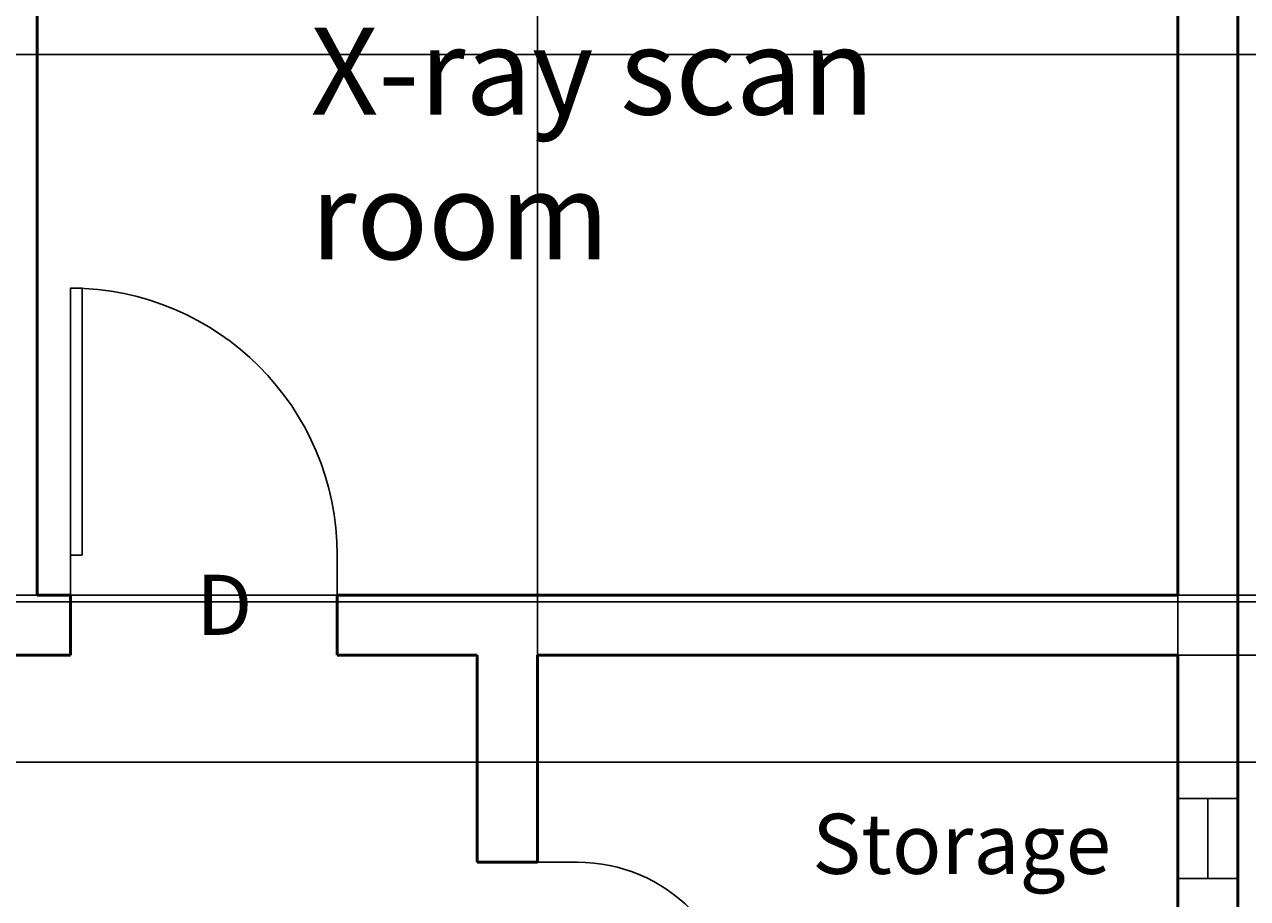
# Model space of a CAD drawing. Units: inches. Extents: x -364 to 705, y -52 to 1250.
# Tile 31 of 34: x 366 to 549, y 786 to 917. Entities that reach past the tile are written whole.
import ezdxf

# ---------------------------------------------------------------- set-up
doc = ezdxf.new("R2010")
doc.units = ezdxf.units.IN
doc.header["$MEASUREMENT"] = 0
for name, color, linetype, lineweight in [('A-ANNO-DIMS', 4, 'Continuous', 18), ('A-ANNO-IDEN', 1, 'Continuous', 18), ('A-AREA-IDEN', 3, 'Continuous', 18), ('A-DOOR', 1, 'Continuous', 25), ('A-GLAZ', 4, 'Continuous', 25), ('A-WALL', 41, 'Continuous', 50)]:
    doc.layers.add(name, color=color, linetype=linetype, lineweight=lineweight)
doc.styles.get("Standard").update_dxf_attribs({"font": 'arial.ttf'})
doc.dimstyles.get("Standard").update_dxf_attribs({"dimtxt": 1, "dimasz": 1, "dimexe": 0.18, "dimexo": 0.0625, "dimgap": 0.09, "dimtad": 0, "dimtih": 1, "dimtoh": 1, "dimdec": 0, "dimzin": 0, "dimdsep": 46, "dimlunit": 3, "dimtxsty": 'Standard', "dimcen": 0.09, "dimadec": 0, "dimazin": 0, "dimtfac": 1, "dimtdec": 0, "dimtofl": 0, "dimtmove": 0, "dimatfit": 3, "dimfxl": 1, "dimtolj": 1, "dimtzin": 0, "dimarcsym": 0})

# ---------------------------------------------------------------- blocks, each defined once
blk = doc.blocks.new('*U2')
for p, q in [((0, 0), (0, -6)), ((40, 0), (40, -6))]:
    blk.add_line(p, q)
blk.add_lwpolyline([(0, 0), (0, 40), (1.75, 40), (1.75, 0)], close=True)
blk.add_arc((0, 0), 40, 0, 90)
blk = doc.blocks.new('*U3')
for p, q in [((0, 0), (0, -6)), ((-24, 0), (-24, -6))]:
    blk.add_line(p, q)
blk.add_lwpolyline([(0, 0), (0, 24), (-1.75, 24), (-1.75, 0)], close=True)
blk.add_arc((0, 0), 24, 90, 180)
blk = doc.blocks.new('*D83')
at = {"layer": 'A-ANNO-DIMS', "color": 0, "lineweight": -2, "transparency": 16777216}
for p, q in [((538.64, 822.11), (703.01, 822.11)), ((702.83, 821.11), (702.83, 788.22)), ((702.83, 754.11), (702.83, 787.01)), ((538.64, 753.11), (703.01, 753.11))]:
    blk.add_line(p, q, dxfattribs=at)
at = {"layer": 'A-ANNO-DIMS', "color": 0, "transparency": 16777216}
for points in [[(702.66, 821.11), (703, 821.11), (702.83, 822.11)], [(702.66, 754.11), (703, 754.11), (702.83, 753.11)]]:
    blk.add_solid(points, dxfattribs=at)
at = {"layer": 'Defpoints', "color": 0, "transparency": 16777216}
for p in [(538.58, 822.11), (702.83, 822.11), (538.58, 753.11)]:
    blk.add_point(p, dxfattribs=at)
at = {"layer": 'A-ANNO-DIMS', "color": 0, "transparency": 16777216, "insert": (702.83, 787.61), "char_height": 1, "attachment_point": 5}
blk.add_mtext('\\A1;5\'-9"', dxfattribs=at)
blk = doc.blocks.new('*D84')
at = {"layer": 'A-ANNO-DIMS', "color": 0, "lineweight": -2, "transparency": 16777216}
for p, q in [((547.64, 986.11), (703.01, 986.11)), ((702.83, 985.11), (702.83, 904.72)), ((702.83, 823.11), (702.83, 903.51)), ((538.64, 822.11), (703.01, 822.11))]:
    blk.add_line(p, q, dxfattribs=at)
at = {"layer": 'A-ANNO-DIMS', "color": 0, "transparency": 16777216}
for points in [[(702.66, 985.11), (703, 985.11), (702.83, 986.11)], [(702.66, 823.11), (703, 823.11), (702.83, 822.11)]]:
    blk.add_solid(points, dxfattribs=at)
at = {"layer": 'Defpoints', "color": 0, "transparency": 16777216}
for p in [(547.58, 986.11), (702.83, 986.11), (538.58, 822.11)]:
    blk.add_point(p, dxfattribs=at)
at = {"layer": 'A-ANNO-DIMS', "color": 0, "transparency": 16777216, "insert": (702.83, 904.11), "char_height": 1, "attachment_point": 5}
blk.add_mtext('\\A1;13\'-8"', dxfattribs=at)
blk = doc.blocks.new('*D97')
at = {"layer": 'A-ANNO-DIMS', "color": 0, "lineweight": -2, "transparency": 16777216}
for p, q in [((358.64, 912.11), (703.01, 912.11)), ((702.83, 911.11), (702.83, 872.22)), ((702.83, 832.11), (702.83, 871.01)), ((358.64, 831.11), (703.01, 831.11))]:
    blk.add_line(p, q, dxfattribs=at)
at = {"layer": 'A-ANNO-DIMS', "color": 0, "transparency": 16777216}
for points in [[(702.66, 911.11), (703, 911.11), (702.83, 912.11)], [(702.66, 832.11), (703, 832.11), (702.83, 831.11)]]:
    blk.add_solid(points, dxfattribs=at)
at = {"layer": 'Defpoints', "color": 0, "transparency": 16777216}
for p in [(358.58, 912.11), (358.58, 831.11), (702.83, 831.11)]:
    blk.add_point(p, dxfattribs=at)
at = {"layer": 'A-ANNO-DIMS', "color": 0, "transparency": 16777216, "insert": (702.83, 871.61), "char_height": 1, "attachment_point": 5}
blk.add_mtext('\\A1;6\'-9"', dxfattribs=at)
blk = doc.blocks.new('*D99')
at = {"layer": 'A-ANNO-DIMS', "color": 0, "lineweight": -2, "transparency": 16777216}
for p, q in [((442.58, 822.18), (442.58, 1141.54)), ((443.58, 1141.36), (489.16, 1141.36)), ((537.58, 1141.36), (492, 1141.36)), ((538.58, 822.18), (538.58, 1141.54))]:
    blk.add_line(p, q, dxfattribs=at)
at = {"layer": 'A-ANNO-DIMS', "color": 0, "transparency": 16777216}
for points in [[(443.58, 1141.53), (443.58, 1141.2), (442.58, 1141.36)], [(537.58, 1141.53), (537.58, 1141.2), (538.58, 1141.36)]]:
    blk.add_solid(points, dxfattribs=at)
at = {"layer": 'Defpoints', "color": 0, "transparency": 16777216}
for p in [(538.58, 1141.36), (442.58, 822.11), (538.58, 822.11)]:
    blk.add_point(p, dxfattribs=at)
at = {"layer": 'A-ANNO-DIMS', "color": 0, "transparency": 16777216, "insert": (490.58, 1141.36), "char_height": 1, "attachment_point": 5}
blk.add_mtext('\\A1;8\'-0"', dxfattribs=at)
blk = doc.blocks.new('*D105')
at = {"layer": 'A-ANNO-DIMS', "color": 0, "lineweight": -2, "transparency": 16777216}
for p, q in [((148.64, 830.11), (703.01, 830.11)), ((702.83, 829.11), (702.83, 818.72)), ((702.83, 807.11), (702.83, 817.51)), ((148.64, 806.11), (703.01, 806.11))]:
    blk.add_line(p, q, dxfattribs=at)
at = {"layer": 'A-ANNO-DIMS', "color": 0, "transparency": 16777216}
for points in [[(702.66, 829.11), (703, 829.11), (702.83, 830.11)], [(702.66, 807.11), (703, 807.11), (702.83, 806.11)]]:
    blk.add_solid(points, dxfattribs=at)
at = {"layer": 'Defpoints', "color": 0, "transparency": 16777216}
for p in [(148.58, 830.11), (148.58, 806.11), (702.83, 806.11)]:
    blk.add_point(p, dxfattribs=at)
at = {"layer": 'A-ANNO-DIMS', "color": 0, "transparency": 16777216, "insert": (702.83, 818.11), "char_height": 1, "attachment_point": 5}
blk.add_mtext('\\A1;2\'-0"', dxfattribs=at)

msp = doc.modelspace()

# ---------------------------------------------------------------- linework, layer by layer
at = {"layer": 'A-GLAZ'}
msp.add_line((543.08, 800.66), (543.08, 788.66), dxfattribs=at)
msp.add_lwpolyline([(538.58, 800.66), (538.58, 788.66), (547.58, 788.66), (547.58, 800.66)], close=True, dxfattribs=at)
at = {"layer": 'A-WALL'}
for p, q in [((547.58, 11.11), (547.58, 986.11)), ((367.58, 831.11), (367.58, 977.11)), ((538.58, 831.11), (538.58, 977.11)), ((372.58, 831.11), (367.58, 831.11)), ((372.58, 822.11), (372.58, 831.11)), ((538.58, 831.11), (412.58, 831.11)), ((412.58, 831.11), (412.58, 822.11)), ((372.58, 822.11), (222.58, 822.11)), ((433.58, 822.11), (412.58, 822.11)), ((433.58, 791.11), (433.58, 822.11)), ((538.58, 822.11), (442.58, 822.11)), ((442.58, 791.11), (442.58, 822.11)), ((538.58, 762.11), (538.58, 822.11)), ((442.58, 791.11), (433.58, 791.11))]:
    msp.add_line(p, q, dxfattribs=at)

# ---------------------------------------------------------------- block references
at = {"layer": 'A-DOOR'}
msp.add_blockref('*U2', (372.58, 837.11), dxfattribs=at)
at = {"layer": 'A-DOOR', "rotation": 270}
msp.add_blockref('*U3', (448.58, 767.11), dxfattribs=at)

# ---------------------------------------------------------------- texts
at = {"layer": 'A-ANNO-IDEN', "insert": (391.42, 834.17), "char_height": 9, "attachment_point": 1}
msp.add_mtext_dynamic_manual_height_columns('D', width=17.6397, gutter_width=1, heights=[0], dxfattribs=at)
at = {"layer": 'A-AREA-IDEN', "attachment_point": 1}
for s, width, heights, insert, char_height in [('X-ray scan room', 119.5086, [34.88], (408.58, 916.12), 13), ('Storage', 25.6333, [0.118], (483.79, 798.36), 9)]:
    msp.add_mtext_dynamic_manual_height_columns(s, width=width, gutter_width=1, heights=heights, dxfattribs=dict(at, insert=insert, char_height=char_height))

# ---------------------------------------------------------------- dimensions: what is measured, and where the dimension line sits
at = {"layer": 'A-ANNO-DIMS'}
dim = msp.add_linear_dim(base=(538.58, 1141.36), p1=(442.58, 822.11), p2=(538.58, 822.11), dimstyle='Standard', override={"dimdec": 1, "dimlfac": 1, "dimrnd": 0, "dimzin": 1, "dimdsep": 46, "dimlunit": 4, "dimfrac": 2}, dxfattribs=at)
dim.commit()
dim.dimension.update_dxf_attribs({"geometry": '*D99', "text_midpoint": (490.58, 1141.36)})
for base, p1, p2, picture, middle in [((702.83, 986.11), (538.58, 822.11), (547.58, 986.11), '*D84', (702.83, 904.11)), ((702.83, 831.11), (358.58, 912.11), (358.58, 831.11), '*D97', (702.83, 871.61)), ((702.83, 806.11), (148.58, 830.11), (148.58, 806.11), '*D105', (702.83, 818.11)), ((702.83, 822.11), (538.58, 753.11), (538.58, 822.11), '*D83', (702.83, 787.61))]:
    dim = msp.add_linear_dim(base=base, p1=p1, p2=p2, angle=90, dimstyle='Standard', override={"dimdec": 1, "dimlfac": 1, "dimrnd": 0, "dimzin": 1, "dimdsep": 46, "dimlunit": 4, "dimfrac": 2}, dxfattribs=at)
    dim.commit()
    dim.dimension.update_dxf_attribs({"geometry": picture, "text_midpoint": middle})

doc.saveas('drawing.dxf')
